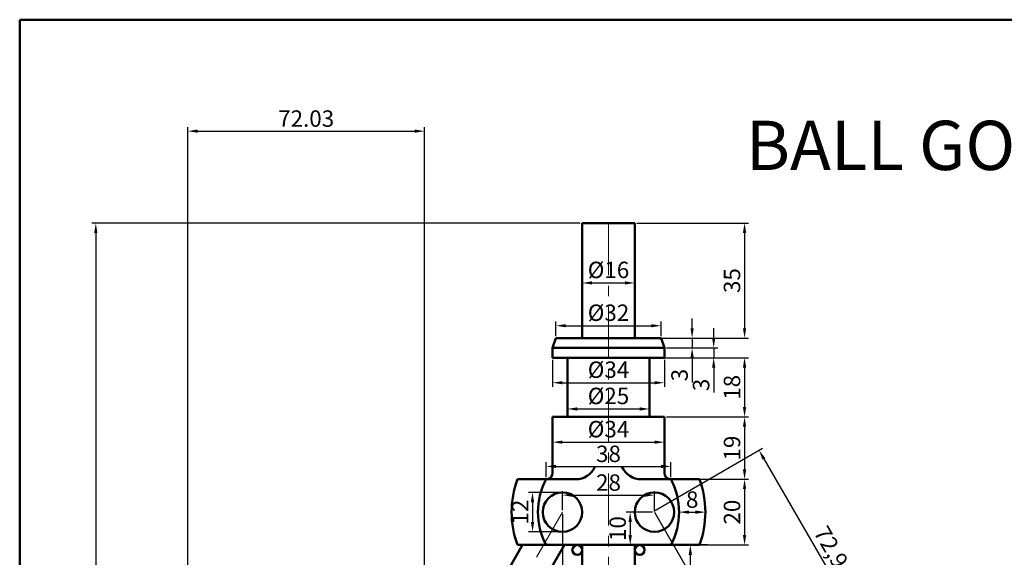
# Model space of a CAD drawing. Units: millimetres. Extents: x 98 to 674, y 38 to 476.
# Tile 6 of 7: x 98 to 398, y 312 to 476. Entities that reach past the tile are written whole.
import ezdxf

# ---------------------------------------------------------------- set-up
doc = ezdxf.new("R2010")
doc.units = ezdxf.units.MM
doc.header["$LTSCALE"] = 0.5
doc.linetypes.add('CENTER', pattern=[50.8, 31.75, -6.35, 6.35, -6.35])
doc.linetypes.add('DASHED', pattern=[19.05, 12.7, -6.35])
for name, color, linetype, lineweight in [('M-CNTR', 1, 'CENTER', 18), ('M-DIMS', 2, 'Continuous', 25), ('M-OUTL', 7, 'Continuous', 50), ('M-PHAN', 6, 'DASHED', 25), ('M-TEXT', 3, 'Continuous', 25), ('M-TTLB', 7, 'Continuous', 50)]:
    doc.layers.add(name, color=color, linetype=linetype, lineweight=lineweight)
doc.styles.get("Standard").update_dxf_attribs({"font": 'arial.ttf'})
doc.dimstyles.new('ISO-25', dxfattribs={"dimtxt": 5, "dimasz": 3, "dimexe": 1.25, "dimexo": 0.625, "dimtad": 1, "dimtxsty": 'Standard', "dimcen": 2.5, "dimadec": 0, "dimazin": 0, "dimtfac": 1, "dimtmove": 0, "dimatfit": 3, "dimfxl": 1, "dimarcsym": 0})

# ---------------------------------------------------------------- blocks, each defined once
blk = doc.blocks.new('*D1')
at = {"layer": 'Defpoints', "color": 0, "ltscale": 0.5, "transparency": 16777216}
for p in [(269.37, 413.69), (285.37, 413.69), (285.37, 395.47)]:
    blk.add_point(p, dxfattribs=at)
at = {"layer": 'M-DIMS', "color": 0, "lineweight": -2, "ltscale": 0.5, "transparency": 16777216}
for p, q in [((269.37, 413.06), (269.37, 394.22)), ((285.37, 413.06), (285.37, 394.22)), ((272.37, 395.47), (282.37, 395.47))]:
    blk.add_line(p, q, dxfattribs=at)
at = {"layer": 'M-DIMS', "color": 0, "ltscale": 0.5, "transparency": 16777216}
for points in [[(272.37, 395.97), (272.37, 394.97), (269.37, 395.47)], [(282.37, 395.97), (282.37, 394.97), (285.37, 395.47)]]:
    blk.add_solid(points, dxfattribs=at)
at = {"layer": 'M-DIMS', "color": 0, "ltscale": 0.5, "transparency": 16777216, "insert": (277.37, 398.79), "char_height": 5, "attachment_point": 5}
blk.add_mtext('%%C16', dxfattribs=at)
blk = doc.blocks.new('*D2')
at = {"layer": 'Defpoints', "color": 0, "ltscale": 0.5, "transparency": 16777216}
for p in [(293.37, 382.45), (261.37, 378.69), (293.37, 378.69)]:
    blk.add_point(p, dxfattribs=at)
at = {"layer": 'M-DIMS', "color": 0, "lineweight": -2, "ltscale": 0.5, "transparency": 16777216}
for p, q in [((261.37, 379.31), (261.37, 383.7)), ((293.37, 379.31), (293.37, 383.7)), ((264.37, 382.45), (290.37, 382.45))]:
    blk.add_line(p, q, dxfattribs=at)
at = {"layer": 'M-DIMS', "color": 0, "ltscale": 0.5, "transparency": 16777216}
for points in [[(264.37, 382.95), (264.37, 381.95), (261.37, 382.45)], [(290.37, 382.95), (290.37, 381.95), (293.37, 382.45)]]:
    blk.add_solid(points, dxfattribs=at)
at = {"layer": 'M-DIMS', "color": 0, "ltscale": 0.5, "transparency": 16777216, "insert": (277.37, 385.76), "char_height": 5, "attachment_point": 5}
blk.add_mtext('%%C32', dxfattribs=at)
blk = doc.blocks.new('*D3')
at = {"layer": 'Defpoints', "color": 0, "ltscale": 0.5, "transparency": 16777216}
for p in [(260.37, 372.69), (294.37, 372.69), (294.37, 365.09)]:
    blk.add_point(p, dxfattribs=at)
at = {"layer": 'M-DIMS', "color": 0, "lineweight": -2, "ltscale": 0.5, "transparency": 16777216}
for p, q in [((260.37, 372.06), (260.37, 363.84)), ((294.37, 372.06), (294.37, 363.84)), ((263.37, 365.09), (291.37, 365.09))]:
    blk.add_line(p, q, dxfattribs=at)
at = {"layer": 'M-DIMS', "color": 0, "ltscale": 0.5, "transparency": 16777216}
for points in [[(263.37, 365.59), (263.37, 364.59), (260.37, 365.09)], [(291.37, 365.59), (291.37, 364.59), (294.37, 365.09)]]:
    blk.add_solid(points, dxfattribs=at)
at = {"layer": 'M-DIMS', "color": 0, "ltscale": 0.5, "transparency": 16777216, "insert": (277.37, 368.41), "char_height": 5, "attachment_point": 5}
blk.add_mtext('%%C34', dxfattribs=at)
blk = doc.blocks.new('*D4')
at = {"layer": 'Defpoints', "color": 0, "ltscale": 0.5, "transparency": 16777216}
for p in [(260.37, 351.72), (294.37, 351.72), (294.37, 347)]:
    blk.add_point(p, dxfattribs=at)
at = {"layer": 'M-DIMS', "color": 0, "lineweight": -2, "ltscale": 0.5, "transparency": 16777216}
for p, q in [((260.37, 351.09), (260.37, 345.75)), ((294.37, 351.09), (294.37, 345.75)), ((263.37, 347), (291.37, 347))]:
    blk.add_line(p, q, dxfattribs=at)
at = {"layer": 'M-DIMS', "color": 0, "ltscale": 0.5, "transparency": 16777216}
for points in [[(263.37, 347.5), (263.37, 346.5), (260.37, 347)], [(291.37, 347.5), (291.37, 346.5), (294.37, 347)]]:
    blk.add_solid(points, dxfattribs=at)
at = {"layer": 'M-DIMS', "color": 0, "ltscale": 0.5, "transparency": 16777216, "insert": (277.37, 350.31), "char_height": 5, "attachment_point": 5}
blk.add_mtext('%%C34', dxfattribs=at)
blk = doc.blocks.new('*D5')
at = {"layer": 'Defpoints', "color": 0, "ltscale": 0.5, "transparency": 16777216}
for p in [(264.87, 357.8), (289.87, 357.8), (289.87, 357.1)]:
    blk.add_point(p, dxfattribs=at)
at = {"layer": 'M-DIMS', "color": 0, "lineweight": -2, "ltscale": 0.5, "transparency": 16777216}
for p, q in [((264.87, 357.18), (264.87, 355.85)), ((267.87, 357.1), (286.87, 357.1)), ((289.87, 357.18), (289.87, 355.85))]:
    blk.add_line(p, q, dxfattribs=at)
at = {"layer": 'M-DIMS', "color": 0, "ltscale": 0.5, "transparency": 16777216}
for points in [[(267.87, 357.6), (267.87, 356.6), (264.87, 357.1)], [(286.87, 357.6), (286.87, 356.6), (289.87, 357.1)]]:
    blk.add_solid(points, dxfattribs=at)
at = {"layer": 'M-DIMS', "color": 0, "ltscale": 0.5, "transparency": 16777216, "insert": (277.37, 360.42), "char_height": 5, "attachment_point": 5}
blk.add_mtext('%%C25', dxfattribs=at)
blk = doc.blocks.new('*D6')
at = {"layer": 'Defpoints', "color": 0, "ltscale": 0.5, "transparency": 16777216}
for p in [(296.37, 339.61), (258.37, 335.69), (296.37, 335.69)]:
    blk.add_point(p, dxfattribs=at)
at = {"layer": 'M-DIMS', "color": 0, "lineweight": -2, "ltscale": 0.5, "transparency": 16777216}
for p, q in [((258.37, 336.31), (258.37, 340.86)), ((261.37, 339.61), (293.37, 339.61)), ((296.37, 336.31), (296.37, 340.86))]:
    blk.add_line(p, q, dxfattribs=at)
at = {"layer": 'M-DIMS', "color": 0, "ltscale": 0.5, "transparency": 16777216}
for points in [[(261.37, 340.11), (261.37, 339.11), (258.37, 339.61)], [(293.37, 340.11), (293.37, 339.11), (296.37, 339.61)]]:
    blk.add_solid(points, dxfattribs=at)
at = {"layer": 'M-DIMS', "color": 0, "ltscale": 0.5, "transparency": 16777216, "insert": (277.37, 342.79), "char_height": 5, "attachment_point": 5}
blk.add_mtext('38', dxfattribs=at)
blk = doc.blocks.new('*D7')
at = {"layer": 'Defpoints', "color": 0, "ltscale": 0.5, "transparency": 16777216}
for p in [(291.37, 330.86), (263.37, 325.69), (291.37, 325.69)]:
    blk.add_point(p, dxfattribs=at)
at = {"layer": 'M-DIMS', "color": 0, "lineweight": -2, "ltscale": 0.5, "transparency": 16777216}
for p, q in [((263.37, 326.31), (263.37, 332.11)), ((266.37, 330.86), (288.37, 330.86)), ((291.37, 326.31), (291.37, 332.11))]:
    blk.add_line(p, q, dxfattribs=at)
at = {"layer": 'M-DIMS', "color": 0, "ltscale": 0.5, "transparency": 16777216}
for points in [[(266.37, 331.36), (266.37, 330.36), (263.37, 330.86)], [(288.37, 331.36), (288.37, 330.36), (291.37, 330.86)]]:
    blk.add_solid(points, dxfattribs=at)
at = {"layer": 'M-DIMS', "color": 0, "ltscale": 0.5, "transparency": 16777216, "insert": (277.37, 334.04), "char_height": 5, "attachment_point": 5}
blk.add_mtext('28', dxfattribs=at)
blk = doc.blocks.new('*D8')
at = {"layer": 'Defpoints', "color": 0, "ltscale": 0.5, "transparency": 16777216}
for p in [(263.37, 331.69), (254.25, 319.69), (263.37, 319.69)]:
    blk.add_point(p, dxfattribs=at)
at = {"layer": 'M-DIMS', "color": 0, "lineweight": -2, "ltscale": 0.5, "transparency": 16777216}
for p, q in [((262.74, 331.69), (253, 331.69)), ((254.25, 328.69), (254.25, 322.69)), ((262.74, 319.69), (253, 319.69))]:
    blk.add_line(p, q, dxfattribs=at)
at = {"layer": 'M-DIMS', "color": 0, "ltscale": 0.5, "transparency": 16777216}
for points in [[(253.75, 328.69), (254.75, 328.69), (254.25, 331.69)], [(253.75, 322.69), (254.75, 322.69), (254.25, 319.69)]]:
    blk.add_solid(points, dxfattribs=at)
at = {"layer": 'M-DIMS', "color": 0, "ltscale": 0.5, "transparency": 16777216, "insert": (251.12, 325.69), "char_height": 5, "attachment_point": 5, "rotation": 90}
blk.add_mtext('12', dxfattribs=at)
blk = doc.blocks.new('*D9')
at = {"layer": 'Defpoints', "color": 0, "ltscale": 0.5, "transparency": 16777216}
for p in [(291.37, 325.69), (283.98, 315.69), (291.37, 315.69)]:
    blk.add_point(p, dxfattribs=at)
at = {"layer": 'M-DIMS', "color": 0, "lineweight": -2, "ltscale": 0.5, "transparency": 16777216}
for p, q in [((290.74, 325.69), (282.73, 325.69)), ((283.98, 322.69), (283.98, 318.69)), ((290.74, 315.69), (282.73, 315.69))]:
    blk.add_line(p, q, dxfattribs=at)
at = {"layer": 'M-DIMS', "color": 0, "ltscale": 0.5, "transparency": 16777216}
for points in [[(283.48, 322.69), (284.48, 322.69), (283.98, 325.69)], [(283.48, 318.69), (284.48, 318.69), (283.98, 315.69)]]:
    blk.add_solid(points, dxfattribs=at)
at = {"layer": 'M-DIMS', "color": 0, "ltscale": 0.5, "transparency": 16777216, "insert": (280.8, 320.69), "char_height": 5, "attachment_point": 5, "rotation": 90}
blk.add_mtext('10', dxfattribs=at)
blk = doc.blocks.new('*D10')
at = {"layer": 'Defpoints', "color": 0, "ltscale": 0.5, "transparency": 16777216}
for p in [(303.2, 335.69), (303.2, 315.69), (318.77, 315.69)]:
    blk.add_point(p, dxfattribs=at)
at = {"layer": 'M-DIMS', "color": 0, "lineweight": -2, "ltscale": 0.5, "transparency": 16777216}
for p, q in [((303.83, 335.69), (320.02, 335.69)), ((318.77, 332.69), (318.77, 318.69)), ((303.83, 315.69), (320.02, 315.69))]:
    blk.add_line(p, q, dxfattribs=at)
at = {"layer": 'M-DIMS', "color": 0, "ltscale": 0.5, "transparency": 16777216}
for points in [[(318.27, 332.69), (319.27, 332.69), (318.77, 335.69)], [(318.27, 318.69), (319.27, 318.69), (318.77, 315.69)]]:
    blk.add_solid(points, dxfattribs=at)
at = {"layer": 'M-DIMS', "color": 0, "ltscale": 0.5, "transparency": 16777216, "insert": (315.6, 325.69), "char_height": 5, "attachment_point": 5, "rotation": 90}
blk.add_mtext('20', dxfattribs=at)
blk = doc.blocks.new('*D11')
at = {"layer": 'Defpoints', "color": 0, "ltscale": 0.5, "transparency": 16777216}
for p in [(298.84, 325.69), (306.84, 325.69), (306.84, 325.69)]:
    blk.add_point(p, dxfattribs=at)
at = {"layer": 'M-DIMS', "color": 0, "lineweight": -2, "ltscale": 0.5, "transparency": 16777216}
for p, q in [((298.84, 325.06), (298.84, 324.44)), ((301.84, 325.69), (303.84, 325.69)), ((306.84, 325.06), (306.84, 324.44))]:
    blk.add_line(p, q, dxfattribs=at)
at = {"layer": 'M-DIMS', "color": 0, "ltscale": 0.5, "transparency": 16777216}
for points in [[(301.84, 326.19), (301.84, 325.19), (298.84, 325.69)], [(303.84, 326.19), (303.84, 325.19), (306.84, 325.69)]]:
    blk.add_solid(points, dxfattribs=at)
at = {"layer": 'M-DIMS', "color": 0, "ltscale": 0.5, "transparency": 16777216, "insert": (302.84, 328.86), "char_height": 5, "attachment_point": 5}
blk.add_mtext('8', dxfattribs=at)
blk = doc.blocks.new('*D12')
at = {"layer": 'Defpoints', "color": 0, "ltscale": 0.5, "transparency": 16777216}
for p in [(294.37, 354.69), (311.93, 335.69), (318.77, 335.69)]:
    blk.add_point(p, dxfattribs=at)
at = {"layer": 'M-DIMS', "color": 0, "lineweight": -2, "ltscale": 0.5, "transparency": 16777216}
for p, q in [((294.99, 354.69), (320.02, 354.69)), ((318.77, 351.69), (318.77, 338.69)), ((312.55, 335.69), (320.02, 335.69))]:
    blk.add_line(p, q, dxfattribs=at)
at = {"layer": 'M-DIMS', "color": 0, "ltscale": 0.5, "transparency": 16777216}
for points in [[(318.27, 351.69), (319.27, 351.69), (318.77, 354.69)], [(318.27, 338.69), (319.27, 338.69), (318.77, 335.69)]]:
    blk.add_solid(points, dxfattribs=at)
at = {"layer": 'M-DIMS', "color": 0, "ltscale": 0.5, "transparency": 16777216, "insert": (315.6, 345.19), "char_height": 5, "attachment_point": 5, "rotation": 90}
blk.add_mtext('19', dxfattribs=at)
blk = doc.blocks.new('*D13')
at = {"layer": 'Defpoints', "color": 0, "ltscale": 0.5, "transparency": 16777216}
for p in [(289.87, 372.69), (294.37, 354.69), (318.77, 354.69)]:
    blk.add_point(p, dxfattribs=at)
at = {"layer": 'M-DIMS', "color": 0, "lineweight": -2, "ltscale": 0.5, "transparency": 16777216}
for p, q in [((290.49, 372.69), (320.02, 372.69)), ((318.77, 369.69), (318.77, 357.69)), ((294.99, 354.69), (320.02, 354.69))]:
    blk.add_line(p, q, dxfattribs=at)
at = {"layer": 'M-DIMS', "color": 0, "ltscale": 0.5, "transparency": 16777216}
for points in [[(318.27, 369.69), (319.27, 369.69), (318.77, 372.69)], [(318.27, 357.69), (319.27, 357.69), (318.77, 354.69)]]:
    blk.add_solid(points, dxfattribs=at)
at = {"layer": 'M-DIMS', "color": 0, "ltscale": 0.5, "transparency": 16777216, "insert": (315.6, 363.69), "char_height": 5, "attachment_point": 5, "rotation": 90}
blk.add_mtext('18', dxfattribs=at)
blk = doc.blocks.new('*D14')
at = {"layer": 'Defpoints', "color": 0, "ltscale": 0.5, "transparency": 16777216}
for p in [(294.37, 375.69), (294.37, 372.69), (309.38, 372.69)]:
    blk.add_point(p, dxfattribs=at)
at = {"layer": 'M-DIMS', "color": 0, "lineweight": -2, "ltscale": 0.5, "transparency": 16777216}
for p, q in [((309.38, 378.69), (309.38, 381.69)), ((294.99, 375.69), (310.63, 375.69)), ((309.38, 375.69), (309.38, 372.69)), ((294.99, 372.69), (310.63, 372.69)), ((309.38, 369.69), (309.38, 362.16))]:
    blk.add_line(p, q, dxfattribs=at)
at = {"layer": 'M-DIMS', "color": 0, "ltscale": 0.5, "transparency": 16777216}
for points in [[(308.88, 378.69), (309.88, 378.69), (309.38, 375.69)], [(308.88, 369.69), (309.88, 369.69), (309.38, 372.69)]]:
    blk.add_solid(points, dxfattribs=at)
at = {"layer": 'M-DIMS', "color": 0, "ltscale": 0.5, "transparency": 16777216, "insert": (306.2, 364.42), "char_height": 5, "attachment_point": 5, "rotation": 90}
blk.add_mtext('3', dxfattribs=at)
blk = doc.blocks.new('*D15')
at = {"layer": 'Defpoints', "color": 0, "ltscale": 0.5, "transparency": 16777216}
for p in [(293.37, 378.69), (294.37, 375.69), (302.81, 375.69)]:
    blk.add_point(p, dxfattribs=at)
at = {"layer": 'M-DIMS', "color": 0, "lineweight": -2, "ltscale": 0.5, "transparency": 16777216}
for p, q in [((302.81, 381.69), (302.81, 384.69)), ((293.99, 378.69), (304.06, 378.69)), ((302.81, 378.69), (302.81, 375.69)), ((294.99, 375.69), (304.06, 375.69)), ((302.81, 372.69), (302.81, 365.16))]:
    blk.add_line(p, q, dxfattribs=at)
at = {"layer": 'M-DIMS', "color": 0, "ltscale": 0.5, "transparency": 16777216}
for points in [[(302.31, 381.69), (303.31, 381.69), (302.81, 378.69)], [(302.31, 372.69), (303.31, 372.69), (302.81, 375.69)]]:
    blk.add_solid(points, dxfattribs=at)
at = {"layer": 'M-DIMS', "color": 0, "ltscale": 0.5, "transparency": 16777216, "insert": (299.63, 367.42), "char_height": 5, "attachment_point": 5, "rotation": 90}
blk.add_mtext('3', dxfattribs=at)
blk = doc.blocks.new('*D16')
at = {"layer": 'Defpoints', "color": 0, "ltscale": 0.5, "transparency": 16777216}
for p in [(285.37, 413.69), (285.37, 378.69), (318.77, 378.69)]:
    blk.add_point(p, dxfattribs=at)
at = {"layer": 'M-DIMS', "color": 0, "lineweight": -2, "ltscale": 0.5, "transparency": 16777216}
for p, q in [((285.99, 413.69), (320.02, 413.69)), ((318.77, 410.69), (318.77, 381.69)), ((285.99, 378.69), (320.02, 378.69))]:
    blk.add_line(p, q, dxfattribs=at)
at = {"layer": 'M-DIMS', "color": 0, "ltscale": 0.5, "transparency": 16777216}
for points in [[(318.27, 410.69), (319.27, 410.69), (318.77, 413.69)], [(318.27, 381.69), (319.27, 381.69), (318.77, 378.69)]]:
    blk.add_solid(points, dxfattribs=at)
at = {"layer": 'M-DIMS', "color": 0, "ltscale": 0.5, "transparency": 16777216, "insert": (315.59, 396.19), "char_height": 5, "attachment_point": 5, "rotation": 90}
blk.add_mtext('35', dxfattribs=at)
blk = doc.blocks.new('*D18')
at = {"layer": 'Defpoints', "color": 0, "ltscale": 0.5, "transparency": 16777216}
for p in [(308.14, 315.69), (301.14, 217.69), (302.27, 217.69)]:
    blk.add_point(p, dxfattribs=at)
at = {"layer": 'M-DIMS', "color": 0, "lineweight": -2, "ltscale": 0.5, "transparency": 16777216}
for p, q in [((307.51, 315.69), (301.02, 315.69)), ((302.27, 312.69), (302.27, 220.69)), ((301.76, 217.69), (303.52, 217.69))]:
    blk.add_line(p, q, dxfattribs=at)
at = {"layer": 'M-DIMS', "color": 0, "ltscale": 0.5, "transparency": 16777216}
for points in [[(301.77, 312.69), (302.77, 312.69), (302.27, 315.69)], [(301.77, 220.69), (302.77, 220.69), (302.27, 217.69)]]:
    blk.add_solid(points, dxfattribs=at)
at = {"layer": 'M-DIMS', "color": 0, "ltscale": 0.5, "transparency": 16777216, "insert": (299.09, 266.69), "char_height": 5, "attachment_point": 5, "rotation": 90}
blk.add_mtext('98', dxfattribs=at)
blk = doc.blocks.new('*D20')
at = {"layer": 'Defpoints', "color": 0, "ltscale": 0.5, "transparency": 16777216}
for p in [(290.59, 325.69), (359.62, 281.36), (327.04, 262.55)]:
    blk.add_point(p, dxfattribs=at)
at = {"layer": 'M-DIMS', "color": 0, "lineweight": -2, "ltscale": 0.5, "transparency": 16777216}
for p, q in [((291.13, 326), (324.25, 345.12)), ((324.67, 341.9), (358.12, 283.96)), ((327.58, 262.86), (360.7, 281.99))]:
    blk.add_line(p, q, dxfattribs=at)
at = {"layer": 'M-DIMS', "color": 0, "ltscale": 0.5, "transparency": 16777216}
for points in [[(325.1, 342.15), (324.24, 341.65), (323.17, 344.5)], [(358.56, 284.21), (357.69, 283.71), (359.62, 281.36)]]:
    blk.add_solid(points, dxfattribs=at)
at = {"layer": 'M-DIMS', "color": 0, "ltscale": 0.5, "transparency": 16777216, "insert": (344.54, 314.74), "char_height": 5, "attachment_point": 5, "rotation": 300}
blk.add_mtext('72,9', dxfattribs=at)
blk = doc.blocks.new('*D22')
at = {"layer": 'Defpoints', "color": 0, "ltscale": 0.5, "transparency": 16777216}
for p in [(291.37, 325.69), (378.81, 252.55)]:
    blk.add_point(p, dxfattribs=at)
at = {"layer": 'M-DIMS', "color": 0, "lineweight": -2, "ltscale": 0.5, "transparency": 16777216}
blk.add_line((327.65, 295.34), (376.51, 254.47), dxfattribs=at)
blk.add_arc((291.37, 325.69), 114, 313.9161, 320.7202, dxfattribs=at)
at = {"layer": 'M-DIMS', "color": 0, "ltscale": 0.5, "transparency": 16777216}
blk.add_solid([(376.83, 254.86), (376.19, 254.09), (378.81, 252.55)], dxfattribs=at)
at = {"layer": 'M-DIMS', "color": 0, "ltscale": 0.5, "transparency": 16777216, "insert": (336.2, 292.27), "char_height": 5, "attachment_point": 5, "rotation": 320.0919}
blk.add_mtext('R114', dxfattribs=at)
blk = doc.blocks.new('*D68')
at = {"layer": 'Defpoints', "color": 0, "ltscale": 0.5, "transparency": 16777216}
for p in [(263.37, 325.69), (206.37, 226.96), (263.37, 42.76)]:
    blk.add_point(p, dxfattribs=at)
at = {"layer": 'M-DIMS', "color": 0, "lineweight": -2, "ltscale": 0.5, "transparency": 16777216}
for p, q in [((263.37, 325.06), (263.37, 41.51)), ((206.37, 226.33), (206.37, 41.51)), ((209.37, 42.76), (260.37, 42.76))]:
    blk.add_line(p, q, dxfattribs=at)
at = {"layer": 'M-DIMS', "color": 0, "ltscale": 0.5, "transparency": 16777216}
for points in [[(209.37, 43.26), (209.37, 42.26), (206.37, 42.76)], [(260.37, 43.26), (260.37, 42.26), (263.37, 42.76)]]:
    blk.add_solid(points, dxfattribs=at)
at = {"layer": 'M-DIMS', "color": 0, "ltscale": 0.5, "transparency": 16777216, "insert": (234.87, 45.93), "char_height": 5, "attachment_point": 5}
blk.add_mtext('57', dxfattribs=at)
blk = doc.blocks.new('*D71')
at = {"layer": 'Defpoints', "color": 0, "ltscale": 0.5, "transparency": 16777216}
for p in [(269.37, 413.69), (121.37, 76.69), (269.37, 76.69)]:
    blk.add_point(p, dxfattribs=at)
at = {"layer": 'M-DIMS', "color": 0, "lineweight": -2, "ltscale": 0.5, "transparency": 16777216}
for p, q in [((268.74, 413.69), (120.12, 413.69)), ((121.37, 410.69), (121.37, 79.69)), ((268.74, 76.69), (120.12, 76.69))]:
    blk.add_line(p, q, dxfattribs=at)
at = {"layer": 'M-DIMS', "color": 0, "ltscale": 0.5, "transparency": 16777216}
for points in [[(120.87, 410.69), (121.87, 410.69), (121.37, 413.69)], [(120.87, 79.69), (121.87, 79.69), (121.37, 76.69)]]:
    blk.add_solid(points, dxfattribs=at)
at = {"layer": 'M-DIMS', "color": 0, "ltscale": 0.5, "transparency": 16777216, "insert": (118.19, 245.19), "char_height": 5, "attachment_point": 5, "rotation": 90}
blk.add_mtext('337', dxfattribs=at)
blk = doc.blocks.new('*D73')
at = {"layer": 'Defpoints', "color": 0, "ltscale": 0.5, "transparency": 16777216}
for p in [(221.4, 441.69), (221.4, 168.51), (149.37, 153.69)]:
    blk.add_point(p, dxfattribs=at)
at = {"layer": 'M-DIMS', "color": 0, "lineweight": -2, "ltscale": 0.5, "transparency": 16777216}
for p, q in [((149.37, 154.31), (149.37, 442.94)), ((152.37, 441.69), (218.4, 441.69)), ((221.4, 169.14), (221.4, 442.94))]:
    blk.add_line(p, q, dxfattribs=at)
at = {"layer": 'M-DIMS', "color": 0, "ltscale": 0.5, "transparency": 16777216}
for points in [[(152.37, 442.19), (152.37, 441.19), (149.37, 441.69)], [(218.4, 442.19), (218.4, 441.19), (221.4, 441.69)]]:
    blk.add_solid(points, dxfattribs=at)
at = {"layer": 'M-DIMS', "color": 0, "ltscale": 0.5, "transparency": 16777216, "insert": (185.38, 444.87), "char_height": 5, "attachment_point": 5}
blk.add_mtext('72.03', dxfattribs=at)
blk = doc.blocks.new('*D78')
at = {"layer": 'Defpoints', "color": 0, "ltscale": 0.5, "transparency": 16777216}
for p in [(291.37, 325.69), (348.37, 226.96)]:
    blk.add_point(p, dxfattribs=at)
at = {"layer": 'M-DIMS', "color": 0, "lineweight": -2, "ltscale": 0.5, "transparency": 16777216}
for p, q in [((291.37, 325.69), (348.37, 226.96)), ((386.83, 160.33), (349.87, 224.36))]:
    blk.add_line(p, q, dxfattribs=at)
at = {"layer": 'M-DIMS', "color": 0, "ltscale": 0.5, "transparency": 16777216}
blk.add_solid([(350.3, 224.61), (349.43, 224.11), (348.37, 226.96)], dxfattribs=at)
at = {"layer": 'M-DIMS', "color": 0, "ltscale": 0.5, "transparency": 16777216, "insert": (385.28, 169.29), "char_height": 5, "attachment_point": 5, "rotation": 300.0001}
blk.add_mtext('R114', dxfattribs=at)

msp = doc.modelspace()

# ---------------------------------------------------------------- linework, layer by layer
at = {"layer": 'M-CNTR'}
for p, q in [((277.365, 413.6855), (277.365, 70.7639)), ((263.365, 325.6855), (192.865, 203.5759))]:
    msp.add_line(p, q, dxfattribs=at)
at = {"layer": 'M-OUTL'}
for p, q in [((269.365, 413.6855), (285.365, 413.6855)), ((269.365, 378.6855), (269.365, 413.6855)), ((285.365, 413.6855), (285.365, 378.6855)), ((261.365, 378.6855), (260.365, 375.6855)), ((277.365, 378.6855), (261.365, 378.6855)), ((285.365, 378.6855), (269.365, 378.6855)), ((277.365, 378.6855), (293.365, 378.6855)), ((293.365, 378.6855), (294.365, 375.6855)), ((294.365, 375.6855), (260.365, 375.6855)), ((260.365, 375.6855), (260.365, 372.6855)), ((294.365, 372.6855), (294.365, 375.6855)), ((260.365, 372.6855), (294.365, 372.6855)), ((264.865, 372.6855), (264.865, 354.6855)), ((289.865, 372.6855), (264.865, 372.6855)), ((289.865, 354.6855), (289.865, 372.6855)), ((294.365, 354.6855), (260.365, 354.6855)), ((260.365, 354.6855), (260.365, 337.6855)), ((264.865, 354.6855), (289.865, 354.6855)), ((294.365, 337.6855), (294.365, 354.6855)), ((249.6426, 335.6855), (258.365, 335.6855)), ((258.365, 335.6855), (267.365, 335.6855)), ((287.3523, 335.6855), (296.365, 335.6855)), ((296.365, 335.6855), (305.0875, 335.6855)), ((251.2407, 315.6855), (224.7033, 269.7214)), ((263.9424, 315.6855), (234.5182, 264.7214)), ((305.0875, 315.6855), (249.6426, 315.6855)), ((269.365, 315.6855), (267.865, 315.6855)), ((269.365, 315.6855), (285.365, 315.6855)), ((269.365, 217.6855), (269.365, 315.6855)), ((285.365, 315.6855), (285.365, 217.6855)), ((285.365, 315.6855), (286.865, 315.6855))]:
    msp.add_line(p, q, dxfattribs=at)
for centre, radius in [((263.365, 325.6855), 6), ((291.365, 325.6855), 6), ((267.865, 314.1855), 1.5), ((286.865, 314.1855), 1.5)]:
    msp.add_circle(centre, radius, dxfattribs=at)
for centre, radius, start, end in [((267.3714, 342.1355), 6.4501, 269.943606, 335.909896), ((287.3587, 342.1355), 6.4501, 204.090104, 270.056394), ((277.365, 325.6855), 29.4709, 160.164693, 199.835307), ((277.365, 325.6855), 21.4709, 152.241459, 207.758541), ((258.365, 337.6855), 2, 270, 0), ((296.365, 337.6855), 2, 180, 270), ((277.365, 325.6855), 21.4709, 332.241459, 27.758541), ((277.365, 325.6855), 29.4709, 340.164693, 19.835307)]:
    msp.add_arc(centre, radius, start, end, dxfattribs=at)
at = {"layer": 'M-PHAN'}
msp.add_line((291.365, 325.6855), (375.7053, 179.6039), dxfattribs=at)
at = {"layer": 'M-TTLB', "ltscale": 0.5}
msp.add_lwpolyline([(98.2162, 475.6271), (666.7064, 475.6271), (666.7064, 38.2873), (98.2162, 38.2873)], close=True, dxfattribs=at)

# ---------------------------------------------------------------- texts
at = {"layer": 'M-TEXT', "ltscale": 0.5, "insert": (319.1609, 444.8561), "char_height": 15, "attachment_point": 1}
msp.add_mtext_dynamic_manual_height_columns('BALL GOVERNER', width=187.408111, gutter_width=12.5, heights=[0], dxfattribs=at)

# ---------------------------------------------------------------- dimensions: what is measured, and where the dimension line sits
at = {"layer": 'M-DIMS', "ltscale": 0.5}
for base, p1, p2, override, picture, middle in [((221.3997, 441.6855), (149.365, 153.6855), (221.3997, 168.5142), {"dimdec": 2, "dimlfac": 1, "dimrnd": 0, "dimzin": 0, "dimdsep": 46, "dimlunit": 2}, '*D73', (185.3824, 444.8651)), ((296.365, 339.6082), (258.365, 335.6855), (296.365, 335.6855), {"dimclrd": 0, "dimclre": 0, "dimclrt": 0}, '*D6', (277.365, 342.7878)), ((291.365, 330.8631), (263.365, 325.6855), (291.365, 325.6855), {"dimclrd": 0, "dimclre": 0, "dimclrt": 0}, '*D7', (277.365, 334.041)), ((263.365, 42.7639), (206.365, 226.9586), (263.365, 325.6855), {"dimdec": 0, "dimlfac": 1, "dimrnd": 0, "dimzin": 0, "dimdsep": 46, "dimlunit": 2}, '*D68', (234.865, 45.9316))]:
    dim = msp.add_linear_dim(base=base, p1=p1, p2=p2, dimstyle='ISO-25', override=override, dxfattribs=at)
    dim.commit()
    dim.dimension.update_dxf_attribs({"geometry": picture, "text_midpoint": middle})
for base, p1, p2, override, picture, middle in [((121.365, 76.6855), (269.365, 413.6855), (269.365, 76.6855), {"dimdec": 0, "dimlfac": 1, "dimrnd": 0, "dimzin": 0, "dimdsep": 46, "dimlunit": 2}, '*D71', (118.1855, 245.1855)), ((318.7736, 378.6855), (285.365, 413.6855), (285.365, 378.6855), {"dimclrd": 0, "dimclre": 0, "dimclrt": 0}, '*D16', (315.594, 396.1855)), ((302.8096, 375.6855), (293.365, 378.6855), (294.365, 375.6855), {"dimclrd": 0, "dimclre": 0, "dimclrt": 0}, '*D15', (299.6301, 367.4234)), ((309.3792, 372.6855), (294.365, 375.6855), (294.365, 372.6855), {"dimclrd": 0, "dimclre": 0, "dimclrt": 0}, '*D14', (306.1996, 364.4234)), ((318.7736, 354.6855), (289.865, 372.6855), (294.365, 354.6855), {"dimclrd": 0, "dimclre": 0, "dimclrt": 0}, '*D13', (315.5957, 363.6855)), ((318.7736, 335.6855), (294.365, 354.6855), (311.9254, 335.6855), {"dimclrd": 0, "dimclre": 0, "dimclrt": 0}, '*D12', (315.5957, 345.1855)), ((318.7736, 315.6855), (303.2023, 335.6855), (303.2023, 315.6855), {"dimclrd": 0, "dimclre": 0, "dimclrt": 0}, '*D10', (315.5957, 325.6855)), ((254.2509, 319.6855), (263.365, 331.6855), (263.365, 319.6855), {"dimclrd": 0, "dimclre": 0, "dimclrt": 0}, '*D8', (251.1156, 325.6855)), ((283.9809, 315.6855), (291.365, 325.6855), (291.365, 315.6855), {"dimclrd": 0, "dimclre": 0, "dimclrt": 0}, '*D9', (280.8031, 320.6855)), ((302.2723, 217.6855), (308.1395, 315.6855), (301.1385, 217.6855), {"dimclrd": 0, "dimclre": 0, "dimclrt": 0}, '*D18', (299.0945, 266.6855))]:
    dim = msp.add_linear_dim(base=base, p1=p1, p2=p2, angle=90, dimstyle='ISO-25', override=override, dxfattribs=at)
    dim.commit()
    dim.dimension.update_dxf_attribs({"geometry": picture, "text_midpoint": middle})
for base, p1, p2, picture, middle in [((285.365, 395.4716), (269.365, 413.6855), (285.365, 413.6855), '*D1', (277.365, 398.7893)), ((293.365, 382.4467), (261.365, 378.6855), (293.365, 378.6855), '*D2', (277.365, 385.7644)), ((294.365, 365.091), (260.365, 372.6855), (294.365, 372.6855), '*D3', (277.365, 368.4087)), ((289.865, 357.1026), (264.865, 357.8021), (289.865, 357.8021), '*D5', (277.365, 360.4203)), ((294.365, 346.9972), (260.365, 351.7188), (294.365, 351.7188), '*D4', (277.365, 350.3149))]:
    dim = msp.add_linear_dim(base=base, p1=p1, p2=p2, text='%%C<>', dimstyle='ISO-25', override={"dimclrd": 0, "dimclre": 0, "dimclrt": 0}, dxfattribs=at)
    dim.commit()
    dim.dimension.update_dxf_attribs({"geometry": picture, "text_midpoint": middle})
for p1, p2, distance, picture, middle in [((290.5915, 325.6855), (327.0419, 262.5515), 37.6203, '*D20', (344.5403, 314.7435)), ((298.8359, 325.6855), (306.8359, 325.6855), 0, '*D11', (302.8359, 328.8633))]:
    dim = msp.add_aligned_dim(p1=p1, p2=p2, distance=distance, dimstyle='ISO-25', override={"dimclrd": 0, "dimclre": 0, "dimclrt": 0}, dxfattribs=at)
    dim.commit()
    dim.dimension.update_dxf_attribs({"geometry": picture, "text_midpoint": middle})
for mpoint, override, picture, middle in [((378.8115, 252.5479), {"dimclrd": 0, "dimclre": 0, "dimclrt": 0}, '*D22', (334.1894, 289.8685)), ((348.3652, 226.9587), {"dimdec": 0, "dimlfac": 1, "dimrnd": 0, "dimzin": 0, "dimdsep": 46, "dimlunit": 2}, '*D78', (382.5653, 167.7226))]:
    dim = msp.add_radius_dim(center=(291.365, 325.6855), mpoint=mpoint, dimstyle='ISO-25', override=override, dxfattribs=at)
    dim.commit()
    dim.dimension.update_dxf_attribs({"geometry": picture, "text_midpoint": middle, "dimtype": 164})

doc.saveas('drawing.dxf')
